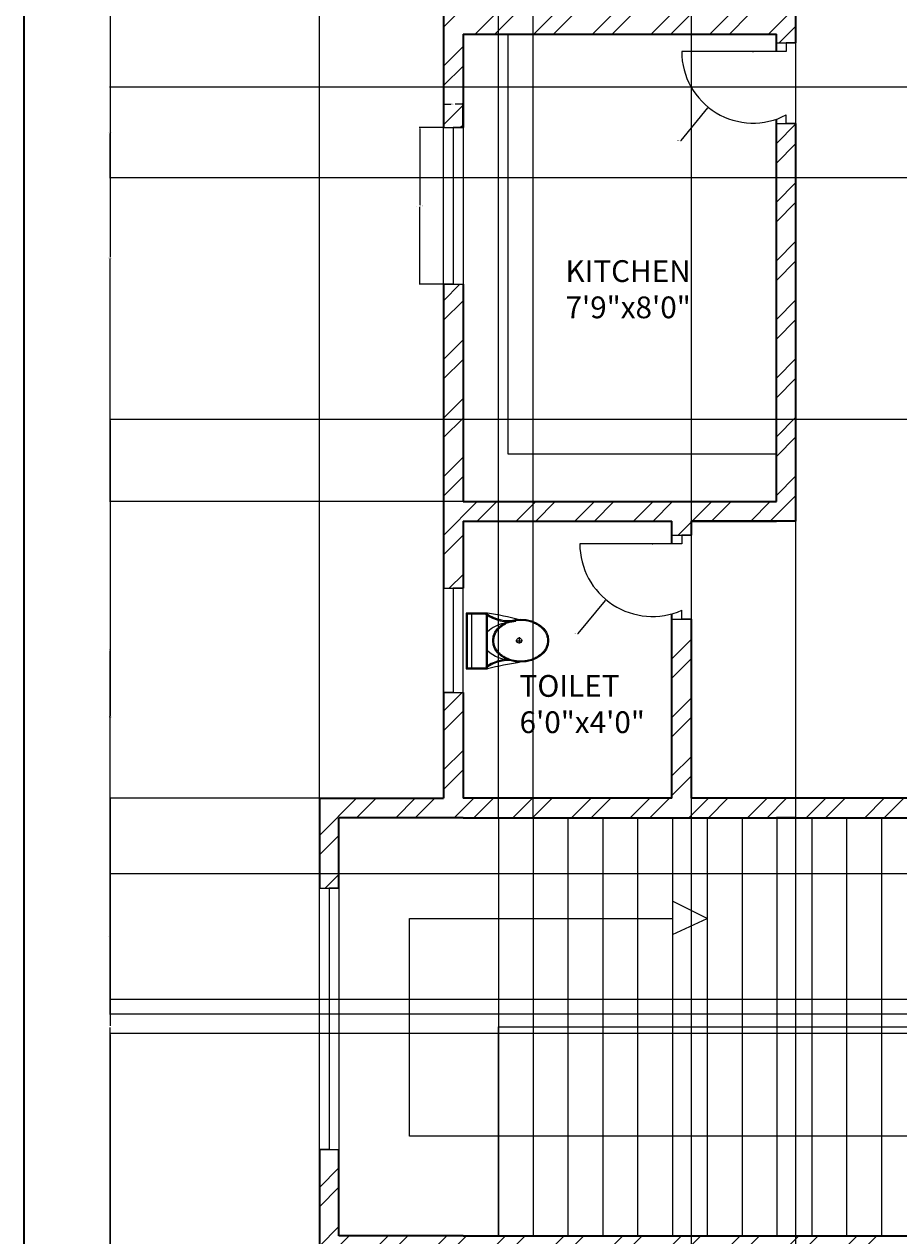
# Model space of a CAD drawing. Units: inches. Extents: x 2008 to 2657, y 1077 to 2165.
# Tile 8 of 16: x 2008 to 2209, y 1567 to 1845. Entities that reach past the tile are written whole.
import ezdxf

# ---------------------------------------------------------------- set-up
doc = ezdxf.new("R2010")
doc.units = ezdxf.units.IN
for name, color, linetype, lineweight in [('A-ANNO-DIMS', 2, 'Continuous', 18), ('A-ANNO-TTLB', 7, 'Continuous', 35), ('A-AREA-IDEN', 4, 'Continuous', 18), ('A-DOOR', 11, 'Continuous', 18), ('A-FLOR-CASE', 9, 'Continuous', 18), ('A-FLOR-FIXT', 8, 'Continuous', 18), ('A-FLOR-STRS', 60, 'Continuous', 18), ('A-GLAZ', 191, 'Continuous', 18), ('A-WALL', 7, 'Continuous', 35)]:
    doc.layers.add(name, color=color, linetype=linetype, lineweight=lineweight)
doc.layers.add('A-WALL-PATT', color=30, linetype='Continuous', lineweight=13, true_color=0xf8991e)
doc.styles.get("Standard").update_dxf_attribs({"font": 'arial.ttf'})
doc.dimstyles.get("Standard").update_dxf_attribs({"dimtxt": 0.18, "dimasz": 0.18, "dimexe": 0.18, "dimexo": 0.0625, "dimgap": 0.09, "dimtad": 0, "dimtih": 1, "dimtoh": 1, "dimdec": 4, "dimzin": 0, "dimdsep": 46, "dimtxsty": 'Standard', "dimcen": 0.09, "dimadec": 0, "dimazin": 0, "dimtfac": 1, "dimtdec": 4, "dimtofl": 0, "dimtmove": 0, "dimatfit": 3, "dimfxl": 1, "dimtolj": 1, "dimtzin": 0, "dimarcsym": 0})

# ---------------------------------------------------------------- blocks, each defined once
blk = doc.blocks.new('A$C31115884')
for p, q in [((283, 498), (223, 498)), ((258, 466), (258, 523)), ((0, 200), (0, 0)), ((520, 200), (0, 200)), ((10, 190), (10, 10)), ((510, 190), (10, 190)), ((510, 10), (510, 190)), ((520, 0), (520, 200)), ((510, 54), (0, 54)), ((10, 10), (510, 10)), ((0, 0), (520, 0))]:
    blk.add_line(p, q)
blk.add_circle((256, 496), 23.6)
for centre, radius, start, end in [((2778, -205), 2807, 165.4549, 171.7133), ((-295, 403), 365, 324.2091, 9.3499), ((-295, 403), 375, 324.2091, 9.3499), ((806, 403), 365, 170.6501, 215.7909), ((3237, 905), 2807, 188.2867, 194.5451), ((384, 406), 293, 190.2774, 224.1564), ((139, 406), 293, 315.8436, 2.6563), ((806, 403), 375, 179.2036, 215.7909)]:
    blk.add_arc(centre, radius, start, end)
blk.add_ellipse((256, 510), major_axis=(0, -261), ratio=0.772727)
blk.add_open_spline([(256, 259), (263, 259), (270, 260), (288, 262), (299, 265), (320, 273), (330, 278), (350, 291), (360, 299), (378, 316), (386, 326), (402, 347), (409, 358), (421, 383), (427, 395), (436, 422), (440, 436), (445, 465), (447, 480), (448, 509), (448, 524), (445, 553), (443, 568), (436, 596), (432, 610), (422, 636), (416, 649), (402, 672), (395, 683), (379, 703), (370, 712), (351, 728), (341, 735), (321, 746), (310, 751), (289, 757), (278, 759), (256, 761), (245, 761), (223, 757), (212, 754), (191, 746), (181, 741), (161, 728), (151, 720), (133, 703), (125, 693), (110, 672), (103, 660), (90, 636), (85, 623), (76, 596), (72, 582), (67, 553), (66, 538), (64, 509), (65, 494), (68, 465), (70, 450), (77, 422), (81, 408), (91, 382), (97, 370), (111, 346), (118, 335), (135, 316), (144, 307), (162, 291), (172, 284), (193, 273), (203, 269), (225, 262), (236, 260), (250, 259), (253, 259), (256, 259)], degree=3, knots=[0, 0, 0, 0, 0.110105, 0.110105, 0.285049, 0.285049, 0.459994, 0.459994, 0.634938, 0.634938, 0.809882, 0.809882, 0.984827, 0.984827, 1.159771, 1.159771, 1.334715, 1.334715, 1.50966, 1.50966, 1.684604, 1.684604, 1.859549, 1.859549, 2.034493, 2.034493, 2.209437, 2.209437, 2.384382, 2.384382, 2.559326, 2.559326, 2.73427, 2.73427, 2.909215, 2.909215, 3.084159, 3.084159, 3.259103, 3.259103, 3.434048, 3.434048, 3.608992, 3.608992, 3.783936, 3.783936, 3.958881, 3.958881, 4.133825, 4.133825, 4.30877, 4.30877, 4.483714, 4.483714, 4.658658, 4.658658, 4.833603, 4.833603, 5.008547, 5.008547, 5.183491, 5.183491, 5.358436, 5.358436, 5.53338, 5.53338, 5.708324, 5.708324, 5.883269, 5.883269, 6.058213, 6.058213, 6.233158, 6.233158, 6.283185, 6.283185, 6.283185, 6.283185])
blk = doc.blocks.new('WIN-24IN-B')
for p, q in [((0, 24), (4.5, 24)), ((0, 24), (0, 0)), ((4.5, 24), (2.25, 24)), ((2.25, 24), (2.25, 0)), ((4.5, 0), (4.5, 24)), ((2.25, 0), (0, 0)), ((0, 0), (4.5, 0))]:
    blk.add_line(p, q)
blk = doc.blocks.new('WIN-36IN-B')
for p, q in [((0, 36), (4.5, 36)), ((0, 0), (0, 36)), ((4.5, 36), (2.25, 36)), ((2.25, 36), (2.25, 0)), ((4.5, 36), (4.5, 0)), ((2.25, 0), (0, 0)), ((0, 0), (4.5, 0))]:
    blk.add_line(p, q)
blk = doc.blocks.new('*D29')
at = {"layer": 'A-ANNO-DIMS', "color": 0, "lineweight": -2, "transparency": 16777216}
for p, q in [((2104.7, 1821.24), (2099.18, 1821.24)), ((2099.36, 1821.06), (2099.36, 1803.42)), ((2099.36, 1785.42), (2099.36, 1803.06)), ((2104.7, 1785.24), (2099.18, 1785.24))]:
    blk.add_line(p, q, dxfattribs=at)
at = {"layer": 'A-ANNO-DIMS', "color": 0, "transparency": 16777216}
for points in [[(2099.33, 1821.06), (2099.39, 1821.06), (2099.36, 1821.24)], [(2099.33, 1785.42), (2099.39, 1785.42), (2099.36, 1785.24)]]:
    blk.add_solid(points, dxfattribs=at)
at = {"layer": 'Defpoints', "color": 0, "transparency": 16777216}
for p in [(2099.36, 1821.24), (2104.76, 1821.24), (2104.76, 1785.24)]:
    blk.add_point(p, dxfattribs=at)
at = {"layer": 'A-ANNO-DIMS', "color": 0, "transparency": 16777216, "insert": (2099.36, 1803.24), "char_height": 0.18, "attachment_point": 5}
blk.add_mtext('\\A1;WIN B 36 TYP.', dxfattribs=at)
blk = doc.blocks.new('*D30')
at = {"layer": 'A-ANNO-DIMS', "color": 0, "lineweight": -2, "transparency": 16777216}
for p, q in [((2104.76, 1821.31), (2104.76, 1826.82)), ((2104.94, 1826.64), (2106.55, 1826.64)), ((2109.08, 1826.64), (2107.47, 1826.64)), ((2109.26, 1821.31), (2109.26, 1826.82))]:
    blk.add_line(p, q, dxfattribs=at)
at = {"layer": 'A-ANNO-DIMS', "color": 0, "transparency": 16777216}
for points in [[(2104.94, 1826.67), (2104.94, 1826.61), (2104.76, 1826.64)], [(2109.08, 1826.67), (2109.08, 1826.61), (2109.26, 1826.64)]]:
    blk.add_solid(points, dxfattribs=at)
at = {"layer": 'Defpoints', "color": 0, "transparency": 16777216}
for p in [(2109.26, 1826.64), (2104.76, 1821.24), (2109.26, 1821.24)]:
    blk.add_point(p, dxfattribs=at)
at = {"layer": 'A-ANNO-DIMS', "color": 0, "transparency": 16777216, "insert": (2107.01, 1826.64), "char_height": 0.18, "attachment_point": 5}
blk.add_mtext('\\A1;5 TYP.', dxfattribs=at)
blk = doc.blocks.new('*D33')
at = {"layer": 'A-ANNO-DIMS', "color": 0, "lineweight": -2, "transparency": 16777216}
for p, q in [((2076.26, 1667.3), (2076.26, 2142.9)), ((2076.44, 2142.72), (2090.19, 2142.72)), ((2104.58, 2142.72), (2090.84, 2142.72)), ((2104.76, 1667.3), (2104.76, 2142.9))]:
    blk.add_line(p, q, dxfattribs=at)
at = {"layer": 'A-ANNO-DIMS', "color": 0, "transparency": 16777216}
for points in [[(2076.44, 2142.75), (2076.44, 2142.69), (2076.26, 2142.72)], [(2104.58, 2142.75), (2104.58, 2142.69), (2104.76, 2142.72)]]:
    blk.add_solid(points, dxfattribs=at)
at = {"layer": 'Defpoints', "color": 0, "transparency": 16777216}
for p in [(2104.76, 2142.72), (2076.26, 1667.24), (2104.76, 1667.24)]:
    blk.add_point(p, dxfattribs=at)
at = {"layer": 'A-ANNO-DIMS', "color": 0, "transparency": 16777216, "insert": (2090.51, 2142.72), "char_height": 0.18, "attachment_point": 5}
blk.add_mtext('\\A1;28.5', dxfattribs=at)
blk = doc.blocks.new('*D43')
at = {"layer": 'A-ANNO-DIMS', "color": 0, "lineweight": -2, "transparency": 16777216}
for p, q in [((2076.2, 1667.24), (2028.03, 1667.24)), ((2028.21, 1667.06), (2028.21, 1614.92)), ((2028.21, 1562.42), (2028.21, 1614.56)), ((2076.2, 1562.24), (2028.03, 1562.24))]:
    blk.add_line(p, q, dxfattribs=at)
at = {"layer": 'A-ANNO-DIMS', "color": 0, "transparency": 16777216}
for points in [[(2028.18, 1667.06), (2028.24, 1667.06), (2028.21, 1667.24)], [(2028.18, 1562.42), (2028.24, 1562.42), (2028.21, 1562.24)]]:
    blk.add_solid(points, dxfattribs=at)
at = {"layer": 'Defpoints', "color": 0, "transparency": 16777216}
for p in [(2028.21, 1667.24), (2076.26, 1667.24), (2076.26, 1562.24)]:
    blk.add_point(p, dxfattribs=at)
at = {"layer": 'A-ANNO-DIMS', "color": 0, "transparency": 16777216, "insert": (2028.21, 1614.74), "char_height": 0.18, "attachment_point": 5}
blk.add_mtext('\\A1;105', dxfattribs=at)
blk = doc.blocks.new('*D44')
at = {"layer": 'A-ANNO-DIMS', "color": 0, "lineweight": -2, "transparency": 16777216}
for p, q in [((2109.2, 1735.34), (2028.03, 1735.34)), ((2028.21, 1735.16), (2028.21, 1701.47)), ((2028.21, 1667.42), (2028.21, 1701.11)), ((2104.7, 1667.24), (2028.03, 1667.24))]:
    blk.add_line(p, q, dxfattribs=at)
at = {"layer": 'A-ANNO-DIMS', "color": 0, "transparency": 16777216}
for points in [[(2028.18, 1735.16), (2028.24, 1735.16), (2028.21, 1735.34)], [(2028.18, 1667.42), (2028.24, 1667.42), (2028.21, 1667.24)]]:
    blk.add_solid(points, dxfattribs=at)
at = {"layer": 'Defpoints', "color": 0, "transparency": 16777216}
for p in [(2028.21, 1735.34), (2109.26, 1735.34), (2104.76, 1667.24)]:
    blk.add_point(p, dxfattribs=at)
at = {"layer": 'A-ANNO-DIMS', "color": 0, "transparency": 16777216, "insert": (2028.21, 1701.29), "char_height": 0.18, "attachment_point": 5}
blk.add_mtext('\\A1;68.1', dxfattribs=at)
blk = doc.blocks.new('*D45')
at = {"layer": 'A-ANNO-DIMS', "color": 0, "lineweight": -2, "transparency": 16777216}
for p, q in [((2109.2, 1847.17), (2028.03, 1847.17)), ((2028.21, 1846.99), (2028.21, 1791.44)), ((2028.21, 1735.52), (2028.21, 1791.08)), ((2109.2, 1735.34), (2028.03, 1735.34))]:
    blk.add_line(p, q, dxfattribs=at)
at = {"layer": 'A-ANNO-DIMS', "color": 0, "transparency": 16777216}
for points in [[(2028.18, 1846.99), (2028.24, 1846.99), (2028.21, 1847.17)], [(2028.18, 1735.52), (2028.24, 1735.52), (2028.21, 1735.34)]]:
    blk.add_solid(points, dxfattribs=at)
at = {"layer": 'Defpoints', "color": 0, "transparency": 16777216}
for p in [(2028.21, 1847.17), (2109.26, 1847.17), (2109.26, 1735.34)]:
    blk.add_point(p, dxfattribs=at)
at = {"layer": 'A-ANNO-DIMS', "color": 0, "transparency": 16777216, "insert": (2028.21, 1791.26), "char_height": 0.18, "attachment_point": 5}
blk.add_mtext('\\A1;111.83', dxfattribs=at)
blk = doc.blocks.new('*D52')
at = {"layer": 'A-ANNO-DIMS', "color": 0, "lineweight": -2, "transparency": 16777216}
for p, q in [((2406.7, 1754.17), (2028.03, 1754.17)), ((2028.21, 1753.99), (2028.21, 1686.11)), ((2028.21, 1617.85), (2028.21, 1685.74)), ((2406.7, 1617.67), (2028.03, 1617.67))]:
    blk.add_line(p, q, dxfattribs=at)
at = {"layer": 'A-ANNO-DIMS', "color": 0, "transparency": 16777216}
for points in [[(2028.18, 1753.99), (2028.24, 1753.99), (2028.21, 1754.17)], [(2028.18, 1617.85), (2028.24, 1617.85), (2028.21, 1617.67)]]:
    blk.add_solid(points, dxfattribs=at)
at = {"layer": 'Defpoints', "color": 0, "transparency": 16777216}
for p in [(2406.76, 1754.17), (2028.21, 1617.67), (2406.76, 1617.67)]:
    blk.add_point(p, dxfattribs=at)
at = {"layer": 'A-ANNO-DIMS', "color": 0, "transparency": 16777216, "insert": (2028.21, 1685.92), "char_height": 0.18, "attachment_point": 5}
blk.add_mtext('\\A1;136.5', dxfattribs=at)
blk = doc.blocks.new('*D53')
at = {"layer": 'A-ANNO-DIMS', "color": 0, "lineweight": -2, "transparency": 16777216}
for p, q in [((2406.7, 1613.17), (2028.03, 1613.17)), ((2028.21, 1612.99), (2028.21, 1545.11)), ((2028.21, 1476.85), (2028.21, 1544.74)), ((2406.7, 1476.67), (2028.03, 1476.67))]:
    blk.add_line(p, q, dxfattribs=at)
at = {"layer": 'A-ANNO-DIMS', "color": 0, "transparency": 16777216}
for points in [[(2028.18, 1612.99), (2028.24, 1612.99), (2028.21, 1613.17)], [(2028.18, 1476.85), (2028.24, 1476.85), (2028.21, 1476.67)]]:
    blk.add_solid(points, dxfattribs=at)
at = {"layer": 'Defpoints', "color": 0, "transparency": 16777216}
for p in [(2406.76, 1613.17), (2028.21, 1476.67), (2406.76, 1476.67)]:
    blk.add_point(p, dxfattribs=at)
at = {"layer": 'A-ANNO-DIMS', "color": 0, "transparency": 16777216, "insert": (2028.21, 1544.92), "char_height": 0.18, "attachment_point": 5}
blk.add_mtext('\\A1;136.5', dxfattribs=at)
blk = doc.blocks.new('*D54')
at = {"layer": 'A-ANNO-DIMS', "color": 0, "lineweight": -2, "transparency": 16777216}
for p, q in [((2161.76, 1514.3), (2161.76, 2142.9)), ((2161.94, 2142.72), (2173.54, 2142.72)), ((2185.58, 2142.72), (2173.98, 2142.72)), ((2185.76, 1514.3), (2185.76, 2142.9))]:
    blk.add_line(p, q, dxfattribs=at)
at = {"layer": 'A-ANNO-DIMS', "color": 0, "transparency": 16777216}
for points in [[(2161.94, 2142.75), (2161.94, 2142.69), (2161.76, 2142.72)], [(2185.58, 2142.75), (2185.58, 2142.69), (2185.76, 2142.72)]]:
    blk.add_solid(points, dxfattribs=at)
at = {"layer": 'Defpoints', "color": 0, "transparency": 16777216}
for p in [(2185.76, 2142.72), (2161.76, 1514.24), (2185.76, 1514.24)]:
    blk.add_point(p, dxfattribs=at)
at = {"layer": 'A-ANNO-DIMS', "color": 0, "transparency": 16777216, "insert": (2173.76, 2142.72), "char_height": 0.18, "attachment_point": 5}
blk.add_mtext('\\A1;24', dxfattribs=at)
blk = doc.blocks.new('*D58')
at = {"layer": 'A-ANNO-DIMS', "color": 0, "lineweight": -2, "transparency": 16777216}
for p, q in [((2459.7, 1830.5), (2028.03, 1830.5)), ((2028.21, 1830.32), (2028.21, 1820.26)), ((2028.21, 1809.84), (2028.21, 1819.9)), ((2459.7, 1809.66), (2028.03, 1809.66))]:
    blk.add_line(p, q, dxfattribs=at)
at = {"layer": 'A-ANNO-DIMS', "color": 0, "transparency": 16777216}
for points in [[(2028.18, 1830.32), (2028.24, 1830.32), (2028.21, 1830.5)], [(2028.18, 1809.84), (2028.24, 1809.84), (2028.21, 1809.66)]]:
    blk.add_solid(points, dxfattribs=at)
at = {"layer": 'Defpoints', "color": 0, "transparency": 16777216}
for p in [(2028.21, 1830.5), (2459.76, 1830.5), (2459.76, 1809.66)]:
    blk.add_point(p, dxfattribs=at)
at = {"layer": 'A-ANNO-DIMS', "color": 0, "transparency": 16777216, "insert": (2028.21, 1820.08), "char_height": 0.18, "attachment_point": 5}
blk.add_mtext('\\A1;20.835', dxfattribs=at)
blk = doc.blocks.new('*D59')
at = {"layer": 'A-ANNO-DIMS', "color": 0, "lineweight": -2, "transparency": 16777216}
for p, q in [((2302.94, 1649.88), (2028.03, 1649.88)), ((2028.21, 1649.7), (2028.21, 1635.62)), ((2028.21, 1621.18), (2028.21, 1635.26)), ((2302.94, 1621), (2028.03, 1621))]:
    blk.add_line(p, q, dxfattribs=at)
at = {"layer": 'A-ANNO-DIMS', "color": 0, "transparency": 16777216}
for points in [[(2028.18, 1649.7), (2028.24, 1649.7), (2028.21, 1649.88)], [(2028.18, 1621.18), (2028.24, 1621.18), (2028.21, 1621)]]:
    blk.add_solid(points, dxfattribs=at)
at = {"layer": 'Defpoints', "color": 0, "transparency": 16777216}
for p in [(2028.21, 1649.88), (2303, 1649.88), (2303, 1621)]:
    blk.add_point(p, dxfattribs=at)
at = {"layer": 'A-ANNO-DIMS', "color": 0, "transparency": 16777216, "insert": (2028.21, 1635.44), "char_height": 0.18, "attachment_point": 5}
blk.add_mtext('\\A1;28.875', dxfattribs=at)
blk = doc.blocks.new('*D63')
at = {"layer": 'A-ANNO-DIMS', "color": 0, "lineweight": -2, "transparency": 16777216}
for p, q in [((2117.38, 1662.8), (2117.38, 2142.9)), ((2117.56, 2142.72), (2121.23, 2142.72)), ((2125.2, 2142.72), (2121.53, 2142.72)), ((2125.38, 1662.8), (2125.38, 2142.9))]:
    blk.add_line(p, q, dxfattribs=at)
at = {"layer": 'A-ANNO-DIMS', "color": 0, "transparency": 16777216}
for points in [[(2117.56, 2142.75), (2117.56, 2142.69), (2117.38, 2142.72)], [(2125.2, 2142.75), (2125.2, 2142.69), (2125.38, 2142.72)]]:
    blk.add_solid(points, dxfattribs=at)
at = {"layer": 'Defpoints', "color": 0, "transparency": 16777216}
for p in [(2125.38, 2142.72), (2117.38, 1662.74), (2125.38, 1662.74)]:
    blk.add_point(p, dxfattribs=at)
at = {"layer": 'A-ANNO-DIMS', "color": 0, "transparency": 16777216, "insert": (2121.38, 2142.72), "char_height": 0.18, "attachment_point": 5}
blk.add_mtext('\\A1;8', dxfattribs=at)
blk = doc.blocks.new('*D87')
at = {"layer": 'A-ANNO-DIMS', "color": 0, "lineweight": -2, "transparency": 16777216}
for p, q in [((2175.82, 1838.68), (2176, 1838.68)), ((2175.91, 1838.59), (2175.91, 1838.77)), ((2159.41, 1818.28), (2165.48, 1825.79)), ((2159.23, 1818.28), (2159.41, 1818.28))]:
    blk.add_line(p, q, dxfattribs=at)
at = {"layer": 'A-ANNO-DIMS', "color": 0, "transparency": 16777216}
blk.add_solid([(2165.46, 1825.81), (2165.51, 1825.77), (2165.6, 1825.93)], dxfattribs=at)
at = {"layer": 'Defpoints', "color": 0, "transparency": 16777216}
for p in [(2175.91, 1838.68), (2165.6, 1825.93)]:
    blk.add_point(p, dxfattribs=at)
at = {"layer": 'A-ANNO-DIMS', "color": 0, "transparency": 16777216, "insert": (2158.82, 1818.28), "char_height": 0.18, "attachment_point": 5}
blk.add_mtext('\\A1;R16.4', dxfattribs=at)
blk = doc.blocks.new('*D89')
at = {"layer": 'A-ANNO-DIMS', "color": 0, "lineweight": -2, "transparency": 16777216}
for p, q in [((2152.7, 1725.64), (2152.88, 1725.64)), ((2152.79, 1725.55), (2152.79, 1725.73)), ((2135.75, 1705.09), (2142.02, 1712.66)), ((2135.57, 1705.09), (2135.75, 1705.09))]:
    blk.add_line(p, q, dxfattribs=at)
at = {"layer": 'A-ANNO-DIMS', "color": 0, "transparency": 16777216}
blk.add_solid([(2142, 1712.68), (2142.05, 1712.64), (2142.14, 1712.8)], dxfattribs=at)
at = {"layer": 'Defpoints', "color": 0, "transparency": 16777216}
for p in [(2152.79, 1725.64), (2142.14, 1712.8)]:
    blk.add_point(p, dxfattribs=at)
at = {"layer": 'A-ANNO-DIMS', "color": 0, "transparency": 16777216, "insert": (2135.09, 1705.09), "char_height": 0.18, "attachment_point": 5}
blk.add_mtext('\\A1;R16.68', dxfattribs=at)

msp = doc.modelspace()

# ---------------------------------------------------------------- hatches: boundary and pattern name
at = {"layer": 'A-WALL-PATT'}
h = msp.add_hatch(dxfattribs=at)
h.set_pattern_fill('ANSI32', color=256)
h.paths.add_polyline_path([(2109.2619, 2094.6743), (2104.7619, 2094.6743), (2104.7619, 2072.1743), (2104.7619, 2021.6151), (2109.2619, 2021.6151), (2109.2619, 2055.6743), (2126.1387, 2055.6743), (2126.1387, 2057.9243), (2126.1387, 2060.1743), (2109.2619, 2060.1743)])
h.paths.add_polyline_path([(2223.2494, 2057.9243), (2223.2494, 2060.1743), (2186.1387, 2060.1743), (2186.1387, 2055.6743), (2223.2494, 2055.6743)])
h.paths.add_polyline_path([(2250.7619, 2072.1743), (2250.7619, 2090.1743), (2250.7619, 2094.6743), (2246.2619, 2094.6743), (2246.2619, 2060.1743), (2242.7242, 2060.1743), (2242.7242, 2055.6743), (2246.2619, 2055.6743), (2246.2619, 1899.6743), (2242.7458, 1899.6743), (2242.7458, 1897.4243), (2242.7458, 1895.1743), (2246.2619, 1895.1743), (2246.2619, 1878.8745), (2248.5119, 1878.8745), (2250.7619, 1878.8745), (2250.7619, 1991.1743), (2250.7619, 2025.6743), (2257.6798, 2025.6743), (2257.6798, 2027.9243), (2257.6798, 2030.1743), (2250.7619, 2030.1743)])
h.paths.add_polyline_path([(2411.2619, 2031.6743), (2409.0119, 2031.6743), (2406.7619, 2031.6743), (2406.7619, 2030.1743), (2322.7619, 2030.1743), (2322.7619, 2053.3443), (2318.2619, 2053.3443), (2318.2619, 2030.1743), (2305.6798, 2030.1743), (2305.6798, 2025.6743), (2318.2619, 2025.6743), (2322.7619, 2025.6743), (2406.7619, 2025.6743), (2406.7619, 1995.6743), (2406.7619, 1847.2677), (2250.7619, 1847.2677), (2250.7619, 1850.9902), (2248.5119, 1850.9902), (2246.2619, 1850.9902), (2246.2619, 1847.1743), (2246.2619, 1842.7677), (2303.0015, 1842.7677), (2303.0015, 1667.2413), (2298.4208, 1667.2413), (2298.4208, 1662.7413), (2303.0015, 1662.7413), (2303.0015, 1649.8758), (2307.5015, 1649.8758), (2307.5015, 1842.7677), (2406.7619, 1842.7677), (2411.2619, 1842.7677), (2411.2619, 1878.6743), (2415.8196, 1878.6743), (2415.8196, 1880.9243), (2415.8196, 1883.1743), (2411.2619, 1883.1743)])
h.paths.add_polyline_path([(2411.2619, 2094.6743), (2406.7619, 2094.6743), (2318.2619, 2094.6743), (2318.2619, 2077.3443), (2322.7619, 2077.3443), (2322.7619, 2090.1743), (2406.7619, 2090.1743), (2406.7619, 2072.1743), (2406.7619, 2067.6743), (2406.7619, 2052.7524), (2411.2619, 2052.7524), (2411.2619, 2055.6743), (2414.9888, 2055.6743), (2414.9888, 2057.9243), (2414.9888, 2060.1743), (2411.2619, 2060.1743), (2411.2619, 2072.1743)])
h.paths.add_polyline_path([(2576.7619, 2072.1743), (2576.7619, 2094.6743), (2572.2619, 2094.6743), (2572.2619, 2060.1743), (2525.8113, 2060.1743), (2525.8113, 2055.6743), (2572.2619, 2055.6743), (2572.2619, 1994.289), (2576.7619, 1994.289)])
h.paths.add_polyline_path([(2465.8113, 2060.1743), (2436.2802, 2060.1743), (2436.2802, 2055.6743), (2465.8113, 2055.6743), (2465.8113, 2057.9243)])
h.paths.add_polyline_path([(2576.7619, 1934.289), (2574.5119, 1934.289), (2572.2619, 1934.289), (2572.2619, 1883.1743), (2447.7027, 1883.1743), (2447.7027, 1878.6743), (2459.7619, 1878.6743), (2459.7619, 1830.4982), (2464.2619, 1830.4982), (2464.2619, 1878.6743), (2572.2619, 1878.6743), (2572.2619, 1868.4883), (2576.7619, 1868.4883)])
h.paths.add_polyline_path([(2576.7619, 1832.4883), (2572.2619, 1832.4883), (2572.2619, 1806.6743), (2464.2619, 1806.6743), (2464.2619, 1809.6629), (2459.7619, 1809.6629), (2459.7619, 1802.1743), (2483.7619, 1802.1743), (2483.7619, 1778.1743), (2488.2619, 1778.1743), (2488.2619, 1802.1743), (2572.2619, 1802.1743), (2572.2619, 1793.6101), (2576.7619, 1793.6101)])
h.paths.add_polyline_path([(2576.7619, 1769.6101), (2572.2619, 1769.6101), (2572.2619, 1754.1743), (2488.2619, 1754.1743), (2488.2619, 1757.2675), (2486.0119, 1757.2675), (2483.7619, 1757.2675), (2483.7619, 1754.1743), (2447.4528, 1754.1743), (2447.4528, 1749.6743), (2483.7619, 1749.6743), (2572.2619, 1749.6743), (2572.2619, 1715.1837), (2576.7619, 1715.1837)])
h.paths.add_polyline_path([(2576.7619, 1655.1837), (2572.2619, 1655.1837), (2572.2619, 1617.6743), (2411.2619, 1617.6743), (2411.2619, 1749.6743), (2414.2827, 1749.6743), (2414.2827, 1754.1743), (2406.7619, 1754.1743), (2406.7619, 1749.6743), (2406.7619, 1617.6743), (2307.5015, 1617.6743), (2307.5015, 1621.0007), (2305.2515, 1621.0007), (2303.0015, 1621.0007), (2303.0015, 1609.6944), (2307.5015, 1609.6944), (2307.5015, 1613.1743), (2406.7619, 1613.1743), (2406.7619, 1476.6743), (2415.532, 1476.6743), (2415.532, 1478.9243), (2415.532, 1481.1743), (2411.2619, 1481.1743), (2411.2619, 1613.1743), (2572.2619, 1613.1743), (2572.2619, 1584.6086), (2576.7619, 1584.6086)])
h.paths.add_polyline_path([(2576.7619, 1524.6086), (2572.2619, 1524.6086), (2572.2619, 1481.1743), (2483.7619, 1481.1743), (2447.5119, 1481.1743), (2447.5119, 1476.6743), (2483.7619, 1476.6743), (2483.7619, 1473.5051), (2488.2619, 1473.5051), (2488.2619, 1476.6743), (2572.2619, 1476.6743), (2572.2619, 1469.5488), (2576.7619, 1469.5488)])
h.paths.add_polyline_path([(2576.7619, 1445.5488), (2572.2619, 1445.5488), (2572.2619, 1428.6743), (2488.2619, 1428.6743), (2488.2619, 1455.6743), (2486.0119, 1455.6743), (2483.7619, 1455.6743), (2483.7619, 1428.6743), (2459.7619, 1428.6743), (2459.7619, 1422.1519), (2464.2619, 1422.1519), (2464.2619, 1424.1743), (2572.2619, 1424.1743), (2572.2619, 1407.5685), (2576.7619, 1407.5685)])
h.paths.add_polyline_path([(2576.7619, 1371.5685), (2572.2619, 1371.5685), (2572.2619, 1352.1743), (2464.2619, 1352.1743), (2464.2619, 1403.1384), (2462.0119, 1403.1384), (2459.7619, 1403.1384), (2459.7619, 1352.1743), (2446.3194, 1352.1743), (2446.3194, 1347.6743), (2572.2619, 1347.6743), (2572.2619, 1321.0291), (2576.7619, 1321.0291)])
h.paths.add_polyline_path([(2462.703, 1227.6743), (2436.0298, 1227.6743), (2436.0298, 1225.4243), (2436.0298, 1223.1743), (2462.703, 1223.1743), (2462.703, 1225.4243)])
h.paths.add_polyline_path([(2576.7619, 1261.0291), (2574.5119, 1261.0291), (2572.2619, 1261.0291), (2572.2619, 1227.6743), (2522.703, 1227.6743), (2522.703, 1223.1743), (2572.2619, 1223.1743), (2572.2619, 1188.6743), (2576.7619, 1188.6743), (2576.7619, 1193.1743), (2576.7619, 1223.1743)])
h.paths.add_polyline_path([(2414.2823, 1227.6743), (2411.2619, 1227.6743), (2411.2619, 1267.1779), (2409.0119, 1267.1779), (2406.7619, 1267.1779), (2406.7619, 1227.6743), (2322.7619, 1227.6743), (2322.7619, 1244.3623), (2318.2619, 1244.3623), (2318.2619, 1223.1743), (2406.7619, 1223.1743), (2406.7619, 1193.1743), (2406.7619, 1188.6743), (2411.2619, 1188.6743), (2411.2619, 1193.1743), (2411.2619, 1223.1743), (2414.2823, 1223.1743)])
h.paths.add_polyline_path([(2411.2619, 1347.6743), (2414.702, 1347.6743), (2414.702, 1349.9243), (2414.702, 1352.1743), (2411.2619, 1352.1743), (2411.2619, 1416.7413), (2307.5015, 1416.7413), (2307.5015, 1579.8489), (2305.2515, 1579.8489), (2303.0015, 1579.8489), (2303.0015, 1566.7413), (2299.2719, 1566.7413), (2299.2719, 1562.2413), (2303.0015, 1562.2413), (2303.0015, 1416.7413), (2246.2619, 1416.7413), (2246.2619, 1409.8616), (2250.7619, 1409.8616), (2250.7619, 1412.2413), (2406.7619, 1412.2413), (2406.7619, 1292.1743), (2304.9703, 1292.1743), (2304.9703, 1287.6743), (2318.2619, 1287.6743), (2318.2619, 1268.3623), (2322.7619, 1268.3623), (2322.7619, 1287.6743), (2406.7619, 1287.6743), (2406.7619, 1285.4748), (2411.2619, 1285.4748)])
h.paths.add_polyline_path([(2109.2619, 1262.7482), (2104.7619, 1262.7482), (2104.7619, 1223.1743), (2104.7619, 1193.1743), (2104.7619, 1188.6743), (2109.2619, 1188.6743), (2109.2619, 1223.1743), (2126.7928, 1223.1743), (2126.7928, 1225.4243), (2126.7928, 1227.6743), (2109.2619, 1227.6743)])
h.paths.add_polyline_path([(2222.3268, 1227.6743), (2186.7928, 1227.6743), (2186.7928, 1223.1743), (2222.3268, 1223.1743)])
h.paths.add_polyline_path([(2250.7619, 1287.6743), (2256.9703, 1287.6743), (2256.9703, 1289.9243), (2256.9703, 1292.1743), (2250.7619, 1292.1743), (2250.7619, 1382.2078), (2248.5119, 1382.2078), (2246.2619, 1382.2078), (2246.2619, 1347.6743), (2246.2619, 1227.6743), (2242.6068, 1227.6743), (2242.6068, 1223.1743), (2246.2619, 1223.1743), (2246.2619, 1188.6743), (2250.7619, 1188.6743), (2250.7619, 1193.1743), (2250.7619, 1227.6743)])
h.paths.add_polyline_path([(2133.2619, 1349.9243), (2133.2619, 1352.1743), (2109.2619, 1352.1743), (2109.2619, 1375.2826), (2104.7619, 1375.2826), (2104.7619, 1322.7482), (2109.2619, 1322.7482), (2109.2619, 1347.6743), (2133.2619, 1347.6743)])
h.paths.add_polyline_path([(2210.2105, 1352.1743), (2161.7619, 1352.1743), (2161.7619, 1412.2413), (2185.7619, 1412.2413), (2185.7619, 1420.1851), (2183.5119, 1420.1851), (2181.2619, 1420.1851), (2181.2619, 1416.7413), (2109.2619, 1416.7413), (2109.2619, 1452.4006), (2104.7619, 1452.4006), (2104.7619, 1399.2826), (2109.2619, 1399.2826), (2109.2619, 1412.2413), (2157.2619, 1412.2413), (2157.2619, 1352.1743), (2154.3383, 1352.1743), (2154.3383, 1347.6743), (2210.2105, 1347.6743)])
h.paths.add_polyline_path([(2185.7619, 1514.2413), (2161.7619, 1514.2413), (2161.7619, 1518.1307), (2159.5119, 1518.1307), (2157.2619, 1518.1307), (2157.2619, 1514.2413), (2109.2619, 1514.2413), (2109.2619, 1528.997), (2107.0119, 1528.997), (2104.7619, 1528.997), (2104.7619, 1488.4006), (2109.2619, 1488.4006), (2109.2619, 1509.7413), (2181.2619, 1509.7413), (2181.2619, 1441.2042), (2185.7619, 1441.2042)])
h.paths.add_polyline_path([(2270.4025, 1566.7413), (2109.2619, 1566.7413), (2080.7619, 1566.7413), (2080.7619, 1586.5643), (2076.2619, 1586.5643), (2076.2619, 1562.2413), (2080.7619, 1562.2413), (2104.7619, 1562.2413), (2104.7619, 1552.997), (2109.2619, 1552.997), (2109.2619, 1562.2413), (2157.2619, 1562.2413), (2157.2619, 1538.2413), (2161.7619, 1538.2413), (2161.7619, 1562.2413), (2205.2619, 1562.2413), (2270.4025, 1562.2413)])
h.paths.add_polyline_path([(2131.6813, 1897.4243), (2131.6813, 1899.6743), (2109.2619, 1899.6743), (2109.2619, 1961.6151), (2104.7619, 1961.6151), (2104.7619, 1886.8042), (2109.2619, 1886.8042), (2109.2619, 1895.1743), (2131.6813, 1895.1743)])
h.paths.add_polyline_path([(2185.7619, 1847.1743), (2161.7619, 1847.1743), (2161.7619, 1895.1743), (2185.7619, 1895.1743), (2211.543, 1895.1743), (2211.543, 1897.4243), (2211.543, 1899.6743), (2154.0916, 1899.6743), (2154.0916, 1897.4243), (2154.0916, 1895.1743), (2157.2619, 1895.1743), (2157.2619, 1847.1743), (2109.2619, 1847.1743), (2109.2619, 1862.8042), (2104.7619, 1862.8042), (2104.7619, 1821.243), (2109.2619, 1821.243), (2109.2619, 1842.6743), (2181.2619, 1842.6743), (2181.2619, 1840.6763), (2185.7619, 1840.6763)])
h.paths.add_polyline_path([(2109.2619, 1785.243), (2104.7619, 1785.243), (2104.7619, 1715.4691), (2109.2619, 1715.4691), (2109.2619, 1730.8423), (2157.2619, 1730.8423), (2157.2619, 1727.6404), (2161.7619, 1727.6404), (2161.7619, 1730.8423), (2185.7619, 1730.8423), (2185.7619, 1822.1438), (2183.5119, 1822.1438), (2181.2619, 1822.1438), (2181.2619, 1735.3423), (2109.2619, 1735.3423)])
h.paths.add_polyline_path([(2109.2619, 1691.4691), (2104.7619, 1691.4691), (2104.7619, 1667.2413), (2076.2619, 1667.2413), (2076.2619, 1646.5643), (2080.7619, 1646.5643), (2080.7619, 1662.7413), (2109.2619, 1662.7413), (2271.4941, 1662.7413), (2271.4941, 1664.9913), (2271.4941, 1667.2413), (2181.2619, 1667.2413), (2161.7619, 1667.2413), (2161.7619, 1708.3752), (2159.5119, 1708.3752), (2157.2619, 1708.3752), (2157.2619, 1667.2413), (2109.2619, 1667.2413)])
h.paths.add_polyline_path([(2233.1467, 1747.4973), (2270.0737, 1747.4973), (2270.0737, 1766.1547), (2233.1467, 1766.1547)], flags=9)

# ---------------------------------------------------------------- linework, layer by layer
at = {"layer": 'A-ANNO-TTLB'}
msp.add_lwpolyline([(2008.4537, 2164.5615), (2657.4477, 2164.5615), (2657.4477, 1076.8888), (2008.4537, 1076.8888)], close=True, dxfattribs=at)
at = {"layer": 'A-DOOR'}
for p, q in [((2181.2619, 1840.6763), (2185.7619, 1840.6763)), ((2185.7619, 1840.6763), (2183.5119, 1840.6763)), ((2183.5119, 1840.6763), (2183.5119, 1838.6763)), ((2183.5119, 1838.6763), (2159.5119, 1838.6763)), ((2183.5119, 1822.1438), (2183.5119, 1824.1438)), ((2181.2619, 1822.1438), (2185.7619, 1822.1438)), ((2185.7619, 1822.1438), (2183.5119, 1822.1438)), ((2159.5119, 1725.6404), (2136.1046, 1725.6404)), ((2157.2619, 1727.6404), (2161.7619, 1727.6404)), ((2161.7619, 1727.6404), (2159.5119, 1727.6404)), ((2159.5119, 1727.6404), (2159.5119, 1725.6404)), ((2157.2619, 1708.3752), (2161.7619, 1708.3752)), ((2159.5119, 1708.3752), (2159.5119, 1710.3752)), ((2161.7619, 1708.3752), (2159.5119, 1708.3752))]:
    msp.add_line(p, q, dxfattribs=at)
for centre, radius, end in [((2175.9118, 1838.6763), 16.3999, 297.608376), ((2152.7859, 1725.6404), 16.6812, 293.778969)]:
    msp.add_arc(centre, radius, 180, end, dxfattribs=at)
at = {"layer": 'A-FLOR-CASE'}
for p, q in [((2119.5946, 1842.6743), (2119.5946, 1746.3001)), ((2119.5946, 1746.3001), (2181.2619, 1746.3001))]:
    msp.add_line(p, q, dxfattribs=at)
at = {"layer": 'A-FLOR-STRS'}
for p, q in [((2117.3789, 1662.7413), (2117.3789, 1566.7413)), ((2125.3789, 1662.7413), (2125.3789, 1566.7413)), ((2133.3789, 1662.7413), (2133.3789, 1566.7413)), ((2141.3789, 1662.7413), (2141.3789, 1566.7413)), ((2149.3789, 1662.7413), (2149.3789, 1566.7413)), ((2157.3789, 1662.7413), (2157.3789, 1566.7413)), ((2165.3789, 1662.7413), (2165.3789, 1566.7413)), ((2173.3789, 1662.7413), (2173.3789, 1566.7413)), ((2181.3789, 1662.7413), (2181.3789, 1566.7413)), ((2189.3789, 1662.7413), (2189.3789, 1566.7413)), ((2197.3789, 1662.7413), (2197.3789, 1566.7413)), ((2205.3789, 1662.7413), (2205.3789, 1566.7413)), ((2165.3789, 1639.6373), (2157.3789, 1643.6)), ((2157.3789, 1643.6), (2157.3789, 1635.8941)), ((2096.9521, 1589.6092), (2096.9521, 1639.6373)), ((2096.9521, 1639.6373), (2157.3789, 1639.6373)), ((2157.3789, 1635.8941), (2165.3789, 1639.6373)), ((2117.3789, 1566.7413), (2117.3789, 1614.7413)), ((2117.3789, 1614.7413), (2237.3789, 1614.7413)), ((2250.4174, 1589.6092), (2096.9521, 1589.6092))]:
    msp.add_line(p, q, dxfattribs=at)
at = {"layer": 'A-GLAZ'}
for p, q in [((2076.2619, 1646.5643), (2080.7619, 1646.5643)), ((2076.2619, 1586.5643), (2076.2619, 1646.5643)), ((2080.7619, 1646.5643), (2078.5119, 1646.5643)), ((2078.5119, 1646.5643), (2078.5119, 1586.5643)), ((2080.7619, 1646.5643), (2080.7619, 1588.9716)), ((2080.7619, 1588.9716), (2080.7619, 1586.5643)), ((2078.5119, 1586.5643), (2076.2619, 1586.5643)), ((2076.2619, 1586.5643), (2080.7619, 1586.5643))]:
    msp.add_line(p, q, dxfattribs=at)
at = {"layer": 'A-WALL'}
for p, q in [((2104.7619, 1862.8042), (2104.7619, 1821.243)), ((2185.7619, 1840.6763), (2185.7619, 1847.1743)), ((2109.2619, 1842.6743), (2181.2619, 1842.6743)), ((2109.2619, 1842.6743), (2109.2619, 1821.243)), ((2181.2619, 1838.6763), (2181.2619, 1842.6743)), ((2181.2619, 1735.3423), (2181.2619, 1823.1737)), ((2185.7619, 1730.8423), (2185.7619, 1822.1438)), ((2104.7619, 1785.243), (2104.7619, 1715.4691)), ((2109.2619, 1785.243), (2109.2619, 1735.3423)), ((2109.2619, 1735.3423), (2181.2619, 1735.3423)), ((2109.2619, 1735.3423), (2181.2619, 1735.3423)), ((2109.2619, 1730.8423), (2157.2619, 1730.8423)), ((2109.2619, 1730.8423), (2109.2619, 1715.4691)), ((2109.2619, 1730.8423), (2109.2619, 1715.4691)), ((2157.2619, 1725.6404), (2157.2619, 1730.8423)), ((2185.7619, 1730.8423), (2161.7619, 1730.8423)), ((2161.7619, 1730.8423), (2181.2619, 1730.8423)), ((2161.7619, 1727.6404), (2161.7619, 1730.8423)), ((2157.2619, 1667.2413), (2157.2619, 1709.5709)), ((2161.7619, 1667.2413), (2161.7619, 1708.3752)), ((2104.7619, 1691.4691), (2104.7619, 1667.2413)), ((2109.2619, 1691.4691), (2109.2619, 1667.2413)), ((2076.2619, 1667.2413), (2104.7619, 1667.2413)), ((2076.2619, 1667.2413), (2076.2619, 1646.5643)), ((2157.2619, 1667.2413), (2109.2619, 1667.2413)), ((2181.2619, 1667.2413), (2161.7619, 1667.2413)), ((2272.573, 1667.2413), (2181.2619, 1667.2413)), ((2109.2619, 1662.7413), (2080.7619, 1662.7413)), ((2080.7619, 1646.5643), (2080.7619, 1662.7413)), ((2109.2619, 1662.7413), (2271.4941, 1662.7413)), ((2185.7619, 1662.7413), (2181.2619, 1662.7413)), ((2076.2619, 1586.5643), (2076.2619, 1562.2413)), ((2080.7619, 1566.7413), (2080.7619, 1586.5643)), ((2109.2619, 1566.7413), (2080.7619, 1566.7413)), ((2109.2619, 1566.7413), (2270.4025, 1566.7413))]:
    msp.add_line(p, q, dxfattribs=at)

# ---------------------------------------------------------------- block references
at = {"layer": 'A-FLOR-FIXT', "xscale": 0.0246256636748975, "yscale": 0.0246256636748975, "zscale": 0.0246256636748975, "rotation": 270}
msp.add_blockref('A$C31115884', (2109.9535, 1709.7185), dxfattribs=at)
at = {"layer": 'A-GLAZ'}
for name, p in [('WIN-36IN-B', (2104.762, 1785.2434)), ('WIN-24IN-B', (2104.762, 1691.4688))]:
    msp.add_blockref(name, p, dxfattribs=at)

# ---------------------------------------------------------------- texts
at = {"layer": 'A-AREA-IDEN', "char_height": 5, "attachment_point": 1}
for s, width, insert in [('KITCHEN\\P7\'9"x8\'0"', 159.531825, (2132.8004, 1790.7831)), ('TOILET\\P6\'0"x4\'0"', 96.666282, (2122.253, 1695.512))]:
    msp.add_mtext_dynamic_manual_height_columns(s, width=width, gutter_width=12.5, heights=[0], dxfattribs=dict(at, insert=insert))

# ---------------------------------------------------------------- dimensions: what is measured, and where the dimension line sits
at = {"layer": 'A-ANNO-DIMS'}
for base, p1, p2, override, picture, middle in [((2104.7619, 2142.7243), (2076.2619, 1667.2413), (2104.7619, 1667.2413), {"dimdec": 1, "dimlfac": 1, "dimrnd": 0, "dimzin": 0, "dimdsep": 46, "dimlunit": 2}, '*D33', (2090.5119, 2142.7243)), ((2125.3789, 2142.7243), (2117.3789, 1662.7413), (2125.3789, 1662.7413), {"dimdec": 0, "dimlfac": 1, "dimrnd": 0, "dimzin": 0, "dimdsep": 46, "dimlunit": 2}, '*D63', (2121.3789, 2142.7243)), ((2185.7619, 2142.7243), (2161.7619, 1514.2413), (2185.7619, 1514.2413), {"dimdec": 0, "dimlfac": 1, "dimrnd": 0, "dimzin": 0, "dimdsep": 46, "dimlunit": 2}, '*D54', (2173.7619, 2142.7243))]:
    dim = msp.add_linear_dim(base=base, p1=p1, p2=p2, dimstyle='Standard', override=override, dxfattribs=at)
    dim.commit()
    dim.dimension.update_dxf_attribs({"geometry": picture, "text_midpoint": middle})
for base, p1, p2, override, picture, middle in [((2028.2119, 1847.1743), (2109.2619, 1735.3423), (2109.2619, 1847.1743), {"dimdec": 2, "dimlfac": 1, "dimrnd": 0, "dimzin": 0, "dimdsep": 46, "dimlunit": 2}, '*D45', (2028.2119, 1791.2583)), ((2028.2119, 1830.4982), (2459.7619, 1809.6629), (2459.7619, 1830.4982), {"dimdec": 3, "dimlfac": 1, "dimrnd": 0, "dimzin": 0, "dimdsep": 46, "dimlunit": 2}, '*D58', (2028.2119, 1820.0806)), ((2028.2119, 1617.6743), (2406.7619, 1754.1743), (2406.7619, 1617.6743), {"dimdec": 1, "dimlfac": 1, "dimrnd": 0, "dimzin": 0, "dimdsep": 46, "dimlunit": 2}, '*D52', (2028.2119, 1685.9243)), ((2028.2119, 1735.3423), (2104.7619, 1667.2413), (2109.2619, 1735.3423), {"dimdec": 1, "dimlfac": 1, "dimrnd": 0, "dimzin": 0, "dimdsep": 46, "dimlunit": 2}, '*D44', (2028.2119, 1701.2918)), ((2028.2119, 1667.2413), (2076.2619, 1562.2413), (2076.2619, 1667.2413), {"dimdec": 0, "dimlfac": 1, "dimrnd": 0, "dimzin": 0, "dimdsep": 46, "dimlunit": 2}, '*D43', (2028.2119, 1614.7413)), ((2028.2119, 1649.8758), (2303.0015, 1621.0007), (2303.0015, 1649.8758), {"dimdec": 3, "dimlfac": 1, "dimrnd": 0, "dimzin": 0, "dimdsep": 46, "dimlunit": 2}, '*D59', (2028.2119, 1635.4382)), ((2028.2119, 1476.6743), (2406.7619, 1613.1743), (2406.7619, 1476.6743), {"dimdec": 1, "dimlfac": 1, "dimrnd": 0, "dimzin": 0, "dimdsep": 46, "dimlunit": 2}, '*D53', (2028.2119, 1544.9243))]:
    dim = msp.add_linear_dim(base=base, p1=p1, p2=p2, angle=90, dimstyle='Standard', override=override, dxfattribs=at)
    dim.commit()
    dim.dimension.update_dxf_attribs({"geometry": picture, "text_midpoint": middle})
for center, mpoint, override, picture, middle in [((2175.9118, 1838.6763), (2165.5968, 1825.9266), {"dimdec": 1, "dimlfac": 1, "dimrnd": 0, "dimzin": 0, "dimdsep": 46, "dimlunit": 2}, '*D87', (2158.8182, 1818.2767)), ((2152.7859, 1725.6404), (2142.1381, 1712.7995), {"dimdec": 2, "dimlfac": 1, "dimrnd": 0, "dimzin": 0, "dimdsep": 46, "dimlunit": 2}, '*D89', (2135.0894, 1705.0949))]:
    dim = msp.add_radius_dim(center=center, mpoint=mpoint, dimstyle='Standard', override=override, dxfattribs=at)
    dim.commit()
    dim.dimension.update_dxf_attribs({"geometry": picture, "text_midpoint": middle, "dimtype": 164})
dim = msp.add_linear_dim(base=(2109.2619004523, 1826.6430171725), p1=(2104.7619004523, 1821.2430171725), p2=(2109.2619004523, 1821.2430171725), text='<> TYP.', dimstyle='Standard', override={"dimdec": 0, "dimlfac": 1, "dimrnd": 0, "dimzin": 0, "dimdsep": 46, "dimlunit": 2}, dxfattribs=at)
dim.commit()
dim.dimension.update_dxf_attribs({"geometry": '*D30', "text_midpoint": (2107.0119004523, 1826.6430171725)})
dim = msp.add_linear_dim(base=(2099.3619, 1821.243), p1=(2104.7619, 1785.243), p2=(2104.7619, 1821.243), angle=90, text='WIN B <> TYP.', dimstyle='Standard', override={"dimdec": 0, "dimlfac": 1, "dimrnd": 0, "dimzin": 0, "dimdsep": 46, "dimlunit": 2}, dxfattribs=at)
dim.commit()
dim.dimension.update_dxf_attribs({"geometry": '*D29', "text_midpoint": (2099.3619, 1803.243)})

doc.saveas('drawing.dxf')
